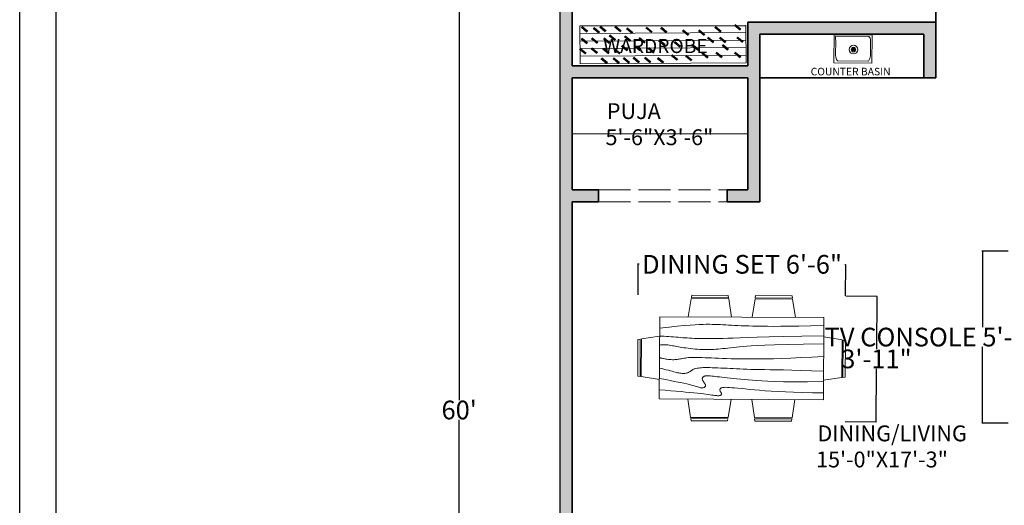
# Model space of a CAD drawing. Units: inches. Extents: x 0 to 4258, y 0 to 3769.
# Tile 19 of 30: x 3476 to 3845, y 3261 to 3443. Entities that reach past the tile are written whole.
import ezdxf

# ---------------------------------------------------------------- set-up
doc = ezdxf.new("R2010")
doc.units = ezdxf.units.IN
doc.header["$MEASUREMENT"] = 0
doc.linetypes.add('ACAD_ISO02W100', pattern=[15, 12, -3])
doc.layers.get('0').update_dxf_attribs({"color": 16})
for name, color, linetype, lineweight in [('A-ANNO-DIMS', 250, 'Continuous', 18), ('A-ANNO-TEXT', 250, 'Continuous', 18), ('A-ANNO-TTLB', 250, 'Continuous', 25), ('A-AREA-IDEN', 250, 'Continuous', 18), ('A-CASE', 150, 'Continuous', 18), ('A-CASE-PATT', 251, 'Continuous', 13), ('A-FLOR-FIXT', 250, 'Continuous', 18), ('A-FLOR-OVHD', 150, 'ACAD_ISO02W100', 13), ('A-WALL-PATT', 16, 'Continuous', 13), ('C-PROP', 150, 'Continuous', 25), ('furniture', 13, 'Continuous', 18), ('walls', 251, 'Continuous', 35)]:
    doc.layers.add(name, color=color, linetype=linetype, lineweight=lineweight)
doc.styles.get("Standard").update_dxf_attribs({"font": 'arial.ttf'})
doc.dimstyles.get("Standard").update_dxf_attribs({"dimtxt": 7, "dimasz": 0.18, "dimexe": 0.18, "dimexo": 0.0625, "dimgap": 0.09, "dimtad": 0, "dimtih": 1, "dimtoh": 1, "dimzin": 0, "dimdsep": 46, "dimlunit": 3, "dimtxsty": 'Standard', "dimcen": 0.09, "dimadec": 0, "dimazin": 0, "dimtfac": 1, "dimtofl": 0, "dimtmove": 0, "dimatfit": 3, "dimfxl": 1, "dimtolj": 1, "dimtzin": 0, "dimarcsym": 0})

# ---------------------------------------------------------------- blocks, each defined once
blk = doc.blocks.new('Dining Set - 36 x 72 in.')
for p, q in [((-22.2343, 26.00059), (-23.4847, 17.99762)), ((-22.2304, 26), (-5.7608, 26)), ((-22, 27.5), (-22.1562, 26.50042)), ((-5.8416, 26.5), (-22.1534, 26.5)), ((-22, 27.5), (-6, 27.5)), ((-5.8437, 26.49966), (-6, 27.5)), ((-4.5152, 17.99762), (-5.7655, 25.99926)), ((5.7657, 26.00059), (4.5153, 17.99762)), ((5.7696, 26), (22.2392, 26)), ((6, 27.5), (5.8438, 26.50042)), ((22.1584, 26.5), (5.8466, 26.5)), ((6, 27.5), (22, 27.5)), ((22.1563, 26.49966), (22, 27.5)), ((23.4848, 17.99762), (22.2345, 25.99926)), ((36, 18), (-36, 18)), ((-36, 18), (-36, -18)), ((36, -18), (36, 18)), ((-44.0006, 8.23428), (-35.9976, 9.48474)), ((44.0006, 8.23428), (35.9976, 9.48474)), ((-45.5, 8), (-44.5004, 8.15617)), ((-45.5, 8), (-45.5, -8)), ((-44.5, -8.15843), (-44.5, 8.15338)), ((-44, 8.23041), (-44, -8.23915)), ((44, 8.23041), (44, -8.23915)), ((44.5, -8.15843), (44.5, 8.15338)), ((45.5, 8), (44.5005, 8.15617)), ((45.5, 8), (45.5, -8)), ((-44.4997, -8.15631), (-45.5, -8)), ((-35.9976, -9.48476), (-43.9993, -8.2345)), ((35.9976, -9.48476), (43.9993, -8.2345)), ((44.4997, -8.15631), (45.5, -8)), ((-36, -18), (36, -18)), ((-22.2343, -26.0006), (-23.4847, -17.99762)), ((-4.5152, -17.99762), (-5.7655, -25.99928)), ((5.7657, -26.0006), (4.5153, -17.99762)), ((23.4848, -17.99762), (22.2345, -25.99928)), ((-22.2304, -26), (-5.7608, -26)), ((-22, -27.5), (-22.1562, -26.50044)), ((-5.8416, -26.5), (-22.1534, -26.5)), ((-22, -27.5), (-6, -27.5)), ((-5.8437, -26.49967), (-6, -27.5)), ((5.7696, -26), (22.2392, -26)), ((6, -27.5), (5.8438, -26.50044)), ((22.1584, -26.5), (5.8466, -26.5)), ((6, -27.5), (22, -27.5)), ((22.1563, -26.49967), (22, -27.5))]:
    blk.add_line(p, q)
for points in [[(-36, 15), (-31.1772, 14.97754), (-26.8079, 14.91406), (-22.8538, 14.81543), (-19.276, 14.6875), (-16.0362, 14.53613), (-13.0957, 14.36718), (-10.4159, 14.18652), (-7.9583, 14), (-5.6904, 13.81315), (-3.6035, 13.63021), (-1.6954, 13.45508), (0.0365, 13.29166), (1.5945, 13.14388), (2.9811, 13.01562), (4.1988, 12.9108), (5.25, 12.83333), (6.1393, 12.78613), (6.8802, 12.76823), (7.4883, 12.77767), (7.9792, 12.8125), (8.3685, 12.87077), (8.6719, 12.95052), (8.9049, 13.0498), (9.0833, 13.16666), (9.2205, 13.29899), (9.3216, 13.44401), (9.3895, 13.59879), (9.4271, 13.76041), (9.4373, 13.92594), (9.4232, 14.09245), (9.3875, 14.257), (9.3333, 14.41666), (9.2638, 14.56917), (9.1836, 14.71484), (9.0975, 14.85465), (9.0104, 14.98958), (8.9272, 15.1206), (8.8529, 15.2487), (8.7922, 15.37483), (8.75, 15.5), (8.7305, 15.62467), (8.7344, 15.74739), (8.7617, 15.86621), (8.8125, 15.97916), (8.8867, 16.08431), (8.9844, 16.17968), (9.1055, 16.26334), (9.25, 16.33333), (9.4189, 16.38802), (9.6172, 16.42708), (9.8506, 16.45052), (10.125, 16.45833), (10.4463, 16.45052), (10.8203, 16.42708), (11.2529, 16.38802), (11.75, 16.33333), (12.3184, 16.26318), (12.9694, 16.17838), (13.7151, 16.07991), (14.5677, 15.96875), (15.5395, 15.84586), (16.6426, 15.71224), (17.8893, 15.56884), (19.2917, 15.41666), (20.859, 15.25667), (22.5879, 15.08984), (24.4721, 14.91715), (26.5052, 14.73958), (28.6809, 14.5581), (30.9929, 14.3737), (33.4347, 14.18733), (36, 14)], [(-36, 10), (-28.9766, 10.14274), (-23.1725, 10.20442), (-18.4241, 10.19775), (-14.5677, 10.13541), (-11.4399, 10.03011), (-8.877, 9.89453), (-6.7154, 9.74137), (-4.7917, 9.58333), (-2.9698, 9.43082), (-1.2246, 9.28515), (0.4415, 9.14534), (2.026, 9.01041), (3.5266, 8.87939), (4.9408, 8.7513), (6.266, 8.62516), (7.5, 8.5), (8.6411, 8.37549), (9.6914, 8.2539), (10.6538, 8.13818), (11.5312, 8.03125), (12.3267, 7.93603), (13.043, 7.85547), (13.6831, 7.79248), (14.25, 7.75), (14.7471, 7.7303), (15.1797, 7.73307), (15.5537, 7.75732), (15.875, 7.80208), (16.1494, 7.86637), (16.3828, 7.94922), (16.5811, 8.04964), (16.75, 8.16666), (16.8944, 8.29915), (17.0143, 8.44531), (17.1089, 8.60319), (17.1771, 8.77083), (17.218, 8.94629), (17.2305, 9.1276), (17.2137, 9.31282), (17.1667, 9.5), (17.0895, 9.6875), (16.987, 9.875), (16.8649, 10.0625), (16.7292, 10.25), (16.5856, 10.4375), (16.4401, 10.625), (16.2985, 10.8125), (16.1667, 11), (16.05, 11.18733), (15.9518, 11.3737), (15.8752, 11.5581), (15.8229, 11.73958), (15.798, 11.91715), (15.8034, 12.08984), (15.842, 12.25667), (15.9167, 12.41666), (16.0295, 12.56836), (16.1784, 12.70833), (16.3605, 12.83268), (16.5729, 12.9375), (16.8127, 13.01888), (17.0768, 13.07291), (17.3625, 13.0957), (17.6667, 13.08333), (17.9894, 13.03312), (18.3418, 12.94726), (18.7382, 12.82918), (19.1927, 12.68229), (19.7195, 12.51001), (20.3327, 12.31575), (21.0465, 12.10294), (21.875, 11.875), (22.8357, 11.63354), (23.959, 11.37304), (25.2786, 11.08618), (26.8282, 10.76562), (28.6414, 10.40405), (30.752, 9.99414), (33.1936, 9.52856), (36, 9)], [(-36, 5.5), (-30.7157, 5.3348), (-26.069, 5.20963), (-21.9946, 5.11767), (-18.4271, 5.05208), (-15.3009, 5.00602), (-12.5508, 4.97265), (-10.1112, 4.94515), (-7.9167, 4.91666), (-5.909, 4.88167), (-4.0586, 4.83984), (-2.3429, 4.79215), (-0.7396, 4.73958), (0.7739, 4.6831), (2.22, 4.6237), (3.6213, 4.56233), (5, 4.5), (6.373, 4.43782), (7.7344, 4.3776), (9.0723, 4.32129), (10.375, 4.27083), (11.6309, 4.22819), (12.8281, 4.19531), (13.9551, 4.17415), (15, 4.16666), (15.954, 4.17448), (16.819, 4.19791), (17.6001, 4.23698), (18.3021, 4.29166), (18.9299, 4.36198), (19.4883, 4.44791), (19.9823, 4.54948), (20.4167, 4.66666), (20.7969, 4.79899), (21.1302, 4.94401), (21.4245, 5.09879), (21.6875, 5.26041), (21.9271, 5.42594), (22.1511, 5.59245), (22.3672, 5.757), (22.5834, 5.91666), (22.8065, 6.06868), (23.0404, 6.21093), (23.2879, 6.34147), (23.5521, 6.45833), (23.8358, 6.55957), (24.142, 6.64323), (24.4735, 6.70735), (24.8334, 6.75), (25.2235, 6.76969), (25.642, 6.76692), (26.0858, 6.74267), (26.5521, 6.69791), (27.0379, 6.63362), (27.5404, 6.55078), (28.0565, 6.45036), (28.5834, 6.33333), (29.1242, 6.19987), (29.7071, 6.04687), (30.3661, 5.87044), (31.1354, 5.66666), (32.0493, 5.43164), (33.142, 5.16146), (34.4475, 4.85221), (36, 4.5)], [(-36, -1), (-30.7915, -0.6591), (-26.0195, -0.38216), (-21.6519, -0.16284), (-17.6563, 0.00521), (-14.0005, 0.12833), (-10.6523, 0.21289), (-7.5796, 0.26522), (-4.75, 0.29166), (-2.134, 0.29793), (0.2878, 0.28711), (2.5317, 0.26163), (4.6146, 0.22396), (6.5529, 0.17651), (8.3633, 0.12174), (10.0623, 0.06209), (11.6667, 0), (13.1899, -0.06201), (14.6341, -0.1211), (15.9982, -0.17432), (17.2813, -0.21875), (18.4823, -0.25147), (19.6003, -0.26953), (20.6343, -0.27002), (21.5834, -0.25), (22.4481, -0.20768), (23.2357, -0.14584), (23.9549, -0.06836), (24.6146, 0.02083), (25.2235, 0.11784), (25.7904, 0.21875), (26.3241, 0.31966), (26.8334, 0.41666), (27.3265, 0.50618), (27.8099, 0.58593), (28.2894, 0.65397), (28.7709, 0.70833), (29.2601, 0.74707), (29.763, 0.76823), (30.2855, 0.76985), (30.8334, 0.75), (31.4088, 0.70784), (31.9994, 0.64713), (32.589, 0.57275), (33.1615, 0.48958), (33.7008, 0.4025), (34.1908, 0.3164), (34.6153, 0.23616), (34.9584, 0.16666), (35.2099, 0.11165), (35.3848, 0.07031), (35.504, 0.04069), (35.5886, 0.02083), (35.6594, 0.00879), (35.7377, 0.0026), (35.8442, 0.00032), (36, 0)], [(-36, -6.5), (-27.1843, -6.31267), (-20.084, -6.1263), (-14.469, -5.9419), (-10.1094, -5.76042), (-6.7752, -5.58285), (-4.2363, -5.41016), (-2.2629, -5.24333), (-0.625, -5.08334), (0.8708, -4.93099), (2.2715, -4.78646), (3.5872, -4.64974), (4.8281, -4.52084), (6.0046, -4.39974), (7.127, -4.28646), (8.2053, -4.18099), (9.25, -4.08334), (10.2705, -3.99382), (11.2734, -3.91407), (12.2647, -3.84603), (13.25, -3.79167), (14.2354, -3.75293), (15.2266, -3.73177), (16.2295, -3.73015), (17.25, -3.75), (18.2912, -3.79248), (19.3451, -3.85547), (20.4009, -3.93604), (21.4479, -4.03125), (22.4754, -4.13819), (23.4727, -4.25391), (24.4289, -4.37549), (25.3334, -4.5), (26.1785, -4.62492), (26.9694, -4.74935), (27.7145, -4.87281), (28.4219, -4.99479), (29.1, -5.11483), (29.7572, -5.23242), (30.4016, -5.34709), (31.0417, -5.45834), (31.6837, -5.56437), (32.3262, -5.65821), (32.9658, -5.73153), (33.599, -5.77604), (34.2224, -5.78345), (34.8327, -5.74545), (35.4264, -5.65373), (36, -5.5)], [(-36, -10), (-26.4022, -9.81299), (-18.4675, -9.62891), (-11.9839, -9.45069), (-6.7396, -9.28125), (-2.5226, -9.12354), (0.8789, -8.98047), (3.6769, -8.85498), (6.0833, -8.75), (8.2767, -8.66765), (10.3021, -8.60677), (12.1712, -8.56543), (13.8958, -8.54167), (15.4876, -8.53353), (16.9583, -8.53907), (18.3197, -8.55632), (19.5834, -8.58334), (20.7616, -8.61841), (21.8685, -8.66081), (22.9188, -8.71004), (23.9271, -8.76563), (24.9081, -8.82707), (25.8763, -8.89388), (26.8465, -8.96558), (27.8334, -9.04167), (28.8474, -9.12118), (29.8828, -9.20117), (30.93, -9.27824), (31.9792, -9.34896), (33.0205, -9.40991), (34.0443, -9.45768), (35.0407, -9.48885), (36, -9.5)], [(-36, -14.5), (-30.0881, -14.33513), (-25.0332, -14.21224), (-20.7312, -14.12647), (-17.0781, -14.07292), (-13.97, -14.04671), (-11.3027, -14.04297), (-8.9724, -14.05681), (-6.875, -14.08334), (-4.9224, -14.11833), (-3.0905, -14.16016), (-1.3709, -14.20785), (0.2448, -14.26042), (1.7647, -14.3169), (3.1973, -14.3763), (4.5507, -14.43767), (5.8333, -14.5), (7.0554, -14.5621), (8.235, -14.62175), (9.3922, -14.67652), (10.5469, -14.72396), (11.7192, -14.76164), (12.929, -14.78711), (14.1965, -14.79794), (15.5417, -14.79167), (16.9933, -14.76424), (18.6152, -14.70508), (20.4804, -14.60197), (22.6615, -14.44271), (25.2312, -14.21509), (28.2624, -13.9069), (31.8277, -13.50594), (36, -13)]]:
    blk.add_lwpolyline(points)
blk = doc.blocks.new('dining area')
at = {"layer": 'furniture', "xscale": 0.6659924291999282, "yscale": 0.6659924291999282, "zscale": 0.6659924291999282, "rotation": 90}
blk.add_blockref('Dining Set - 36 x 72 in.', (-0.44, 20.51), dxfattribs=at)
blk = doc.blocks.new('*D25')
at = {"layer": 'A-ANNO-DIMS', "color": 0, "lineweight": -2, "transparency": 16777216}
for p, q in [((3641.78, 3656.79), (3640.81, 3656.79)), ((3640.99, 3656.61), (3640.99, 3300.46)), ((3640.99, 2936.97), (3640.99, 3293.13)), ((3641.78, 2936.79), (3640.81, 2936.79))]:
    blk.add_line(p, q, dxfattribs=at)
at = {"layer": 'A-ANNO-DIMS', "color": 0, "transparency": 16777216}
for points in [[(3640.96, 3656.61), (3641.02, 3656.61), (3640.99, 3656.79)], [(3640.96, 2936.97), (3641.02, 2936.97), (3640.99, 2936.79)]]:
    blk.add_solid(points, dxfattribs=at)
at = {"layer": 'Defpoints', "color": 0, "transparency": 16777216}
for p in [(3641.85, 3656.79), (3640.99, 2936.79), (3641.85, 2936.79)]:
    blk.add_point(p, dxfattribs=at)
at = {"layer": 'A-ANNO-DIMS', "color": 0, "transparency": 16777216, "insert": (3640.99, 3296.79), "char_height": 7, "attachment_point": 5}
blk.add_mtext("\\A1;60'", dxfattribs=at)
blk = doc.blocks.new('*D38')
at = {"layer": 'A-ANNO-DIMS', "color": 0, "lineweight": -2, "transparency": 16777216}
for p, q in [((3846.84, 3356.33), (3837.06, 3356.33)), ((3837.24, 3356.15), (3837.24, 3327.83)), ((3837.24, 3292.07), (3837.24, 3320.4)), ((3846.84, 3291.89), (3837.06, 3291.89))]:
    blk.add_line(p, q, dxfattribs=at)
at = {"layer": 'A-ANNO-DIMS', "color": 0, "transparency": 16777216}
for points in [[(3837.21, 3356.15), (3837.27, 3356.15), (3837.24, 3356.33)], [(3837.21, 3292.07), (3837.27, 3292.07), (3837.24, 3291.89)]]:
    blk.add_solid(points, dxfattribs=at)
at = {"layer": 'Defpoints', "color": 0, "transparency": 16777216}
for p in [(3837.24, 3356.33), (3846.91, 3356.33), (3846.91, 3291.89)]:
    blk.add_point(p, dxfattribs=at)
at = {"layer": 'A-ANNO-DIMS', "color": 0, "transparency": 16777216, "insert": (3837.24, 3324.11), "char_height": 7, "attachment_point": 5}
blk.add_mtext('\\A1;TV CONSOLE 5\'-4 1/2" TYP.', dxfattribs=at)
blk = doc.blocks.new('*D64')
at = {"layer": 'A-ANNO-DIMS', "color": 0, "lineweight": -2, "transparency": 16777216}
for p, q in [((3708.12, 3339.94), (3708.18, 3351.73)), ((3708.36, 3351.55), (3708.53, 3351.55)), ((3785.82, 3351.18), (3785.65, 3351.18)), ((3785.94, 3339.57), (3786, 3351.36))]:
    blk.add_line(p, q, dxfattribs=at)
at = {"layer": 'A-ANNO-DIMS', "color": 0, "transparency": 16777216}
for points in [[(3708.36, 3351.58), (3708.36, 3351.52), (3708.18, 3351.55)], [(3785.82, 3351.21), (3785.82, 3351.15), (3786, 3351.18)]]:
    blk.add_solid(points, dxfattribs=at)
at = {"layer": 'Defpoints', "color": 0, "transparency": 16777216}
for p in [(3708.18, 3351.55), (3708.12, 3339.88), (3785.94, 3339.51)]:
    blk.add_point(p, dxfattribs=at)
at = {"layer": 'A-ANNO-DIMS', "color": 0, "transparency": 16777216, "insert": (3747.09, 3351.37), "char_height": 7, "attachment_point": 5}
blk.add_mtext('\\A1;DINING SET 6\'-6"', dxfattribs=at)
blk = doc.blocks.new('*D65')
at = {"layer": 'A-ANNO-DIMS', "color": 0, "lineweight": -2, "transparency": 16777216}
for p, q in [((3786, 3339.51), (3797.79, 3339.45)), ((3797.61, 3339.27), (3797.52, 3319.6)), ((3797.39, 3292.59), (3797.48, 3312.27)), ((3785.78, 3292.47), (3797.57, 3292.41))]:
    blk.add_line(p, q, dxfattribs=at)
at = {"layer": 'A-ANNO-DIMS', "color": 0, "transparency": 16777216}
for points in [[(3797.58, 3339.27), (3797.64, 3339.27), (3797.61, 3339.45)], [(3797.36, 3292.6), (3797.42, 3292.59), (3797.39, 3292.41)]]:
    blk.add_solid(points, dxfattribs=at)
at = {"layer": 'Defpoints', "color": 0, "transparency": 16777216}
for p in [(3785.94, 3339.51), (3797.61, 3339.45), (3785.72, 3292.47)]:
    blk.add_point(p, dxfattribs=at)
at = {"layer": 'A-ANNO-DIMS', "color": 0, "transparency": 16777216, "insert": (3797.5, 3315.93), "char_height": 7, "attachment_point": 5}
blk.add_mtext('\\A1;3\'-11"', dxfattribs=at)

msp = doc.modelspace()

# ---------------------------------------------------------------- hatches: boundary and pattern name
at = {"layer": 'A-CASE-PATT'}
h = msp.add_hatch(dxfattribs=at)
h.set_pattern_fill('ANSI31', color=256, scale=0.896631, angle=95.467005, style=0)
h.paths.add_polyline_path([(3688.267, 3430.171), (3686.154, 3431.915), (3686.511, 3432.347), (3688.624, 3430.603)])
h.paths.add_polyline_path([(3696.255, 3426.572), (3694.142, 3428.316), (3694.499, 3428.748), (3696.611, 3427.004)], flags=0)
h.paths.add_polyline_path([(3692.563, 3430.331), (3690.451, 3432.075), (3690.807, 3432.507), (3692.92, 3430.764)], flags=0)
h.paths.add_polyline_path([(3688.872, 3434.025), (3686.76, 3435.768), (3687.116, 3436.2), (3689.229, 3434.457)], flags=0)
h.paths.add_polyline_path([(3700.767, 3426.63), (3698.654, 3428.374), (3699.011, 3428.806), (3701.124, 3427.062)], flags=0)
h.paths.add_polyline_path([(3696.948, 3430.279), (3694.835, 3432.023), (3695.192, 3432.455), (3697.305, 3430.712)], flags=0)
h.paths.add_polyline_path([(3692.654, 3434.047), (3690.541, 3435.79), (3690.898, 3436.223), (3693.01, 3434.479)], flags=0)
h.paths.add_polyline_path([(3688.874, 3438.309), (3686.762, 3440.053), (3687.118, 3440.485), (3689.231, 3438.742)], flags=0)
h.paths.add_polyline_path([(3704.533, 3426.653), (3702.42, 3428.396), (3702.777, 3428.829), (3704.89, 3427.085)], flags=0)
h.paths.add_polyline_path([(3701.103, 3430.175), (3698.991, 3431.918), (3699.347, 3432.35), (3701.46, 3430.607)], flags=0)
h.paths.add_polyline_path([(3697.197, 3434.073), (3695.084, 3435.817), (3695.441, 3436.249), (3697.553, 3434.506)], flags=0)
h.paths.add_polyline_path([(3693.363, 3437.993), (3691.251, 3439.737), (3691.607, 3440.169), (3693.72, 3438.426)], flags=0)
h.paths.add_polyline_path([(3708.246, 3426.807), (3706.133, 3428.55), (3706.49, 3428.982), (3708.602, 3427.239)], flags=0)
h.paths.add_polyline_path([(3703.861, 3431.284), (3701.748, 3433.028), (3702.105, 3433.46), (3704.217, 3431.716)], flags=0)
h.paths.add_polyline_path([(3699.306, 3435.22), (3697.194, 3436.964), (3697.551, 3437.396), (3699.663, 3435.653)], flags=0)
h.paths.add_polyline_path([(3695.749, 3438.439), (3693.636, 3440.183), (3693.993, 3440.615), (3696.106, 3438.871)], flags=0)
h.paths.add_polyline_path([(3712.538, 3426.794), (3710.425, 3428.537), (3710.782, 3428.97), (3712.895, 3427.226)], flags=0)
h.paths.add_polyline_path([(3708.706, 3431.313), (3706.594, 3433.056), (3706.951, 3433.488), (3709.063, 3431.745)], flags=0)
h.paths.add_polyline_path([(3705.04, 3434.846), (3702.927, 3436.59), (3703.284, 3437.022), (3705.397, 3435.278)], flags=0)
h.paths.add_polyline_path([(3701.387, 3438.417), (3699.274, 3440.161), (3699.631, 3440.593), (3701.744, 3438.849)], flags=0)
h.paths.add_polyline_path([(3717.377, 3426.739), (3715.265, 3428.482), (3715.622, 3428.915), (3717.734, 3427.171)], flags=0)
h.paths.add_polyline_path([(3713.853, 3430.44), (3711.741, 3432.184), (3712.097, 3432.616), (3714.21, 3430.872)], flags=0)
h.paths.add_polyline_path([(3710.459, 3434.151), (3708.346, 3435.895), (3708.703, 3436.327), (3710.816, 3434.583)], flags=0)
h.paths.add_polyline_path([(3705.854, 3437.881), (3703.741, 3439.624), (3704.098, 3440.057), (3706.21, 3438.313)], flags=0)
h.paths.add_polyline_path([(3722.656, 3427.808), (3720.544, 3429.552), (3720.9, 3429.984), (3723.013, 3428.241)], flags=0)
h.paths.add_polyline_path([(3717.911, 3433.32), (3715.798, 3435.064), (3716.155, 3435.496), (3718.267, 3433.753)], flags=0)
h.paths.add_polyline_path([(3713.083, 3438.183), (3710.97, 3439.926), (3711.327, 3440.359), (3713.439, 3438.615)], flags=0)
h.paths.add_polyline_path([(3727.976, 3427.58), (3725.863, 3429.323), (3726.22, 3429.756), (3728.333, 3428.012)], flags=0)
h.paths.add_polyline_path([(3723.665, 3432.705), (3721.553, 3434.449), (3721.909, 3434.881), (3724.022, 3433.137)], flags=0)
h.paths.add_polyline_path([(3718.618, 3438.085), (3716.505, 3439.829), (3716.862, 3440.261), (3718.975, 3438.518)], flags=0)
h.paths.add_polyline_path([(3734.113, 3428.633), (3732, 3430.377), (3732.357, 3430.809), (3734.469, 3429.066)], flags=0)
h.paths.add_polyline_path([(3730.557, 3431.441), (3728.444, 3433.184), (3728.801, 3433.616), (3730.913, 3431.873)], flags=0)
h.paths.add_polyline_path([(3726.763, 3437.075), (3724.65, 3438.818), (3725.007, 3439.251), (3727.119, 3437.507)], flags=0)
h.paths.add_polyline_path([(3732.846, 3437.111), (3730.734, 3438.854), (3731.09, 3439.286), (3733.203, 3437.543)], flags=0)
h.paths.add_polyline_path([(3741.617, 3431.506), (3739.505, 3433.249), (3739.862, 3433.681), (3741.974, 3431.938)], flags=0)
h.paths.add_polyline_path([(3736.181, 3434.302), (3734.068, 3436.045), (3734.425, 3436.478), (3736.538, 3434.734)], flags=0)
h.paths.add_polyline_path([(3739.311, 3428.664), (3737.199, 3430.407), (3737.555, 3430.84), (3739.668, 3429.096)], flags=0)
h.paths.add_polyline_path([(3746.28, 3428.705), (3744.167, 3430.448), (3744.524, 3430.88), (3746.636, 3429.137)], flags=0)
h.paths.add_polyline_path([(3747.131, 3434.366), (3745.019, 3436.11), (3745.375, 3436.542), (3747.488, 3434.798)], flags=0)
h.paths.add_polyline_path([(3740.716, 3434.328), (3738.603, 3436.072), (3738.96, 3436.504), (3741.073, 3434.761)], flags=0)
h.paths.add_polyline_path([(3746.324, 3439.073), (3744.212, 3440.817), (3744.568, 3441.249), (3746.681, 3439.506)], flags=0)
h.paths.add_polyline_path([(3738.921, 3438.307), (3736.808, 3440.051), (3737.165, 3440.483), (3739.278, 3438.739)], flags=0)
at = {"layer": 'A-WALL-PATT'}
h = msp.add_hatch(color=256, dxfattribs=at)
h.dxf.hatch_style = 1
h.paths.add_polyline_path([(3753.804, 3425.793), (3753.804, 3437.642), (3815.304, 3437.642), (3815.304, 3421.293), (3819.804, 3421.293), (3819.804, 3442.142), (3749.304, 3442.142), (3749.304, 3425.793), (3683.304, 3425.793), (3683.304, 3652.293), (3773.304, 3652.293), (3773.304, 3638.769), (3777.804, 3638.769), (3777.804, 3656.793), (3678.804, 3656.793), (3678.804, 3163.293), (3711.393, 3163.293), (3711.393, 3167.793), (3683.304, 3167.793), (3683.304, 3374.793), (3693.303, 3374.793), (3693.303, 3379.293), (3683.304, 3379.293), (3683.304, 3421.293), (3749.304, 3421.293), (3749.304, 3379.293), (3741.449, 3379.293), (3741.449, 3374.793), (3753.804, 3374.793)])

# ---------------------------------------------------------------- linework, layer by layer
at = {"layer": 'A-ANNO-TTLB'}
for p, q in [((3476.156, 2762.335), (3476.156, 3768.679)), ((3489.722, 3758.41), (3489.722, 2762.335))]:
    msp.add_line(p, q, dxfattribs=at)
at = {"layer": 'A-CASE'}
for p, q in [((3686.214, 3440.673), (3748.504, 3440.673)), ((3686.23, 3437.844), (3748.518, 3438.209)), ((3686.27, 3440.673), (3686.352, 3426.532)), ((3748.584, 3426.897), (3748.502, 3441.037)), ((3686.247, 3435.016), (3748.535, 3435.381)), ((3686.263, 3432.188), (3748.551, 3432.553)), ((3686.28, 3429.36), (3748.568, 3429.725)), ((3686.297, 3426.532), (3748.584, 3426.897)), ((3683.304, 3400.293), (3749.304, 3400.293))]:
    msp.add_line(p, q, dxfattribs=at)
at = {"layer": 'A-FLOR-FIXT'}
for p, q in [((3781.507, 3427.579), (3781.572, 3437.345)), ((3781.572, 3437.345), (3795.867, 3437.25)), ((3782.212, 3435.347), (3782.174, 3429.574)), ((3782.222, 3436.823), (3794.588, 3436.741)), ((3795.25, 3435.261), (3795.212, 3429.488)), ((3795.867, 3437.25), (3795.798, 3426.777)), ((3788.424, 3432), (3788.181, 3432.291)), ((3788.504, 3432.132), (3788.272, 3432.402)), ((3788.807, 3431.615), (3788.778, 3431.312)), ((3788.89, 3431.299), (3788.926, 3431.599)), ((3789.329, 3431.938), (3789.73, 3432.008)), ((3789.403, 3431.803), (3789.752, 3431.869)), ((3781.503, 3426.871), (3781.507, 3427.579)), ((3782.833, 3427.617), (3794.528, 3427.54)), ((3795.798, 3426.777), (3781.503, 3426.871))]:
    msp.add_line(p, q, dxfattribs=at)
for radius in [1.62, 0.861, 0.507, 0.21]:
    msp.add_circle((3788.893, 3431.806), radius, dxfattribs=at)
for centre, radius, start, end in [((3787.97, 3436.047), 5.8, 172.31244, 186.93184), ((3794, 3435.59), 1.292, 345.23382, 62.92582), ((3785.533, 3429.615), 3.359, 180.69494, 216.4918), ((3791.853, 3429.573), 3.359, 322.75248, 358.54934)]:
    msp.add_arc(centre, radius, start, end, dxfattribs=at)
at = {"layer": 'A-FLOR-OVHD'}
for p, q in [((3693.303, 3379.293), (3741.449, 3379.293)), ((3693.303, 3374.793), (3741.449, 3374.793))]:
    msp.add_line(p, q, dxfattribs=at)
at = {"layer": 'C-PROP'}
msp.add_line((3678.804, 2995.293), (3678.804, 3656.793), dxfattribs=at)
at = {"layer": 'walls'}
for p, q in [((3683.304, 3425.793), (3683.304, 3652.293)), ((3819.804, 3421.293), (3819.804, 3598.293)), ((3749.304, 3425.793), (3749.304, 3442.142)), ((3749.304, 3442.142), (3819.804, 3442.142)), ((3753.804, 3425.793), (3753.804, 3437.658)), ((3753.804, 3437.642), (3815.304, 3437.642)), ((3815.304, 3421.293), (3815.304, 3437.642)), ((3683.304, 3425.793), (3749.304, 3425.793)), ((3753.804, 3374.793), (3753.804, 3425.793)), ((3683.304, 3421.293), (3749.304, 3421.293)), ((3683.304, 3379.293), (3683.304, 3421.293)), ((3749.304, 3379.293), (3749.304, 3421.293)), ((3753.804, 3421.293), (3819.804, 3421.293)), ((3683.304, 3379.293), (3693.303, 3379.293)), ((3693.303, 3379.293), (3693.303, 3374.793)), ((3741.449, 3379.293), (3741.449, 3374.793)), ((3741.449, 3379.293), (3749.304, 3379.293)), ((3683.304, 3374.793), (3693.303, 3374.793)), ((3683.304, 3167.793), (3683.304, 3374.793)), ((3741.449, 3374.793), (3753.804, 3374.793))]:
    msp.add_line(p, q, dxfattribs=at)

# ---------------------------------------------------------------- block references
at = {"layer": 'furniture', "xscale": 1.284087432987447, "yscale": 1.284087432987447, "zscale": 1.284087432987447, "rotation": 89.72449696048554}
msp.add_blockref('dining area', (3773.252, 3316.613), dxfattribs=at)

# ---------------------------------------------------------------- texts
at = {"layer": 'A-ANNO-TEXT'}
for s, height, p in [('WARDROBE', 5.2898, (3695.015, 3430.526)), ('COUNTER BASIN', 2.83673, (3772.83, 3422.167))]:
    msp.add_text(s, height=height, dxfattribs=at).set_placement(p)
at = {"layer": 'A-AREA-IDEN'}
for s, height, p in [('PUJA', 5.939, (3696.366, 3405.804)), ('5\'-6"X3\'-6"', 5.93898, (3695.868, 3396.022)), ('DINING/LIVING', 5.93898, (3775.35, 3285.056)), ('15\'-0"X17\'-3"', 5.93898, (3774.852, 3275.274))]:
    msp.add_text(s, height=height, dxfattribs=at).set_placement(p)

# ---------------------------------------------------------------- dimensions: what is measured, and where the dimension line sits
at = {"layer": 'A-ANNO-DIMS'}
for base, p1, p2, angle, override, picture, middle in [((3640.987, 2936.793), (3641.847, 3656.793), (3641.847, 2936.793), 90, {"dimclrd": 0, "dimclre": 0, "dimclrt": 0}, '*D25', (3640.987, 3296.793)), ((3797.615, 3339.45), (3785.715, 3292.471), (3785.941, 3339.506), 89.7245, {"dimdec": 1, "dimlfac": 1, "dimrnd": 0, "dimzin": 1, "dimdsep": 46, "dimlunit": 4, "dimfrac": 2}, '*D65', (3797.501, 3315.932))]:
    dim = msp.add_linear_dim(base=base, p1=p1, p2=p2, angle=angle, dimstyle='Standard', override=override, dxfattribs=at)
    dim.commit()
    dim.dimension.update_dxf_attribs({"geometry": picture, "text_midpoint": middle})
for base, p1, p2, angle, text, picture, middle in [((3708.176, 3351.554), (3785.941, 3339.506), (3708.12, 3339.88), 179.7245, 'DINING SET <>', '*D64', (3747.087, 3351.366)), ((3837.24, 3356.335), (3846.907, 3291.892), (3846.907, 3356.335), 90, 'TV CONSOLE <> TYP.', '*D38', (3837.24, 3324.113))]:
    dim = msp.add_linear_dim(base=base, p1=p1, p2=p2, angle=angle, text=text, dimstyle='Standard', override={"dimdec": 1, "dimlfac": 1, "dimrnd": 0, "dimzin": 1, "dimdsep": 46, "dimlunit": 4, "dimfrac": 2}, dxfattribs=at)
    dim.commit()
    dim.dimension.update_dxf_attribs({"geometry": picture, "text_midpoint": middle})

doc.saveas('drawing.dxf')
